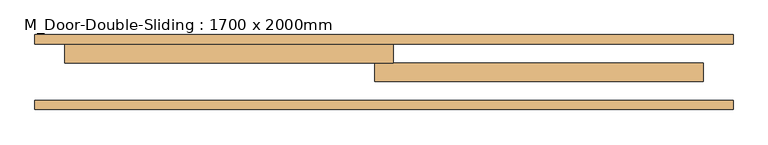
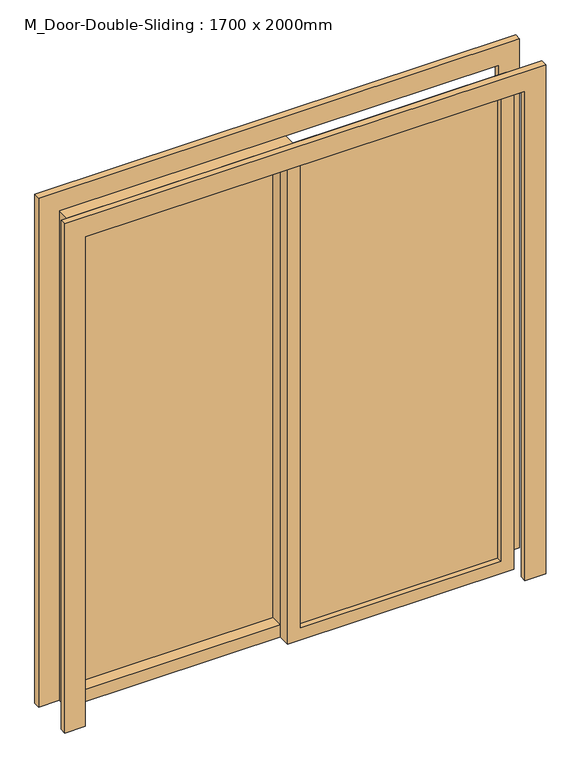
"""IFC4 building model written with IfcOpenShell, lengths in millimetres: door geometry, M_Door-Double-Sliding : 1700 x 2000mm."""

from ifc_helpers import new_model, si_unit, frame, origin, place, context, project, spatial, polyline, outline, extrude, source, transform, mapped, element, save


def m_door_double_sliding_1700_x_2000mm_d36f6dca(model_context):
    return source(origin(), model_context, "Body", "SweptSolid", [
        extrude(outline(polyline([(0.0, 930.0), (2080.0, 930.0), (2080.0, -930.0), (0.0, -930.0), (0.0, -850.0), (2000.0, -850.0), (2000.0, 850.0), (0.0, 850.0), (0.0, 930.0)])), frame((0.0, 202.0, 0.0), z_axis=(0.0, 1.0, 0.0), x_axis=(0.0, 0.0, 1.0)), (0.0, 0.0, 1.0), 25.0),
        extrude(outline(polyline([(0.0, -930.0), (0.0, -850.0), (2000.0, -850.0), (2000.0, 850.0), (0.0, 850.0), (0.0, 930.0), (2080.0, 930.0), (2080.0, -930.0), (0.0, -930.0)])), frame((0.0, 27.0, 0.0), z_axis=(0.0, 1.0, 0.0), x_axis=(0.0, 0.0, 1.0)), (0.0, 0.0, 1.0), 25.0),
        extrude(outline(polyline([(2000.0, 25.0), (2000.0, -850.0), (0.0, -850.0), (0.0, 25.0), (2000.0, 25.0)]), holes=[polyline([(1950.0, -25.0), (50.0, -25.0), (50.0, -800.0), (1950.0, -800.0), (1950.0, -25.0)])]), frame((0.0, 152.0, 0.0), z_axis=(0.0, 1.0, 0.0), x_axis=(0.0, 0.0, 1.0)), (0.0, 0.0, 1.0), 50.0),
        extrude(outline(polyline([(2000.0, -25.0), (0.0, -25.0), (0.0, 850.0), (2000.0, 850.0), (2000.0, -25.0)]), holes=[polyline([(1950.0, 25.0), (1950.0, 800.0), (50.0, 800.0), (50.0, 25.0), (1950.0, 25.0)])]), frame((0.0, 102.0, 0.0), z_axis=(0.0, 1.0, 0.0), x_axis=(0.0, 0.0, 1.0)), (0.0, 0.0, 1.0), 50.0),
        extrude(outline(polyline([(-25.0, 200.025), (-800.0, 200.025), (-800.0, 206.375), (-25.0, 206.375), (-25.0, 200.025)])), frame((0.0, 0.0, 50.0), z_axis=(0.0, 0.0, 1.0), x_axis=(1.0, 0.0, 0.0)), (0.0, 0.0, 1.0), 1900.0),
        extrude(outline(polyline([(25.0, 130.175), (800.0, 130.175), (800.0, 123.825), (25.0, 123.825), (25.0, 130.175)])), frame((0.0, 0.0, 50.0), z_axis=(0.0, 0.0, 1.0), x_axis=(1.0, 0.0, 0.0)), (0.0, 0.0, 1.0), 1900.0),
    ])


if __name__ == "__main__":
    model = new_model("IFC4")
    model_context = context("Model", 3, world=origin())
    ifc_project = project(units=[si_unit("LENGTHUNIT", "METRE", prefix="MILLI")], contexts=[model_context])
    site = spatial("IfcSite", under=ifc_project)
    building = spatial("IfcBuilding", under=site)
    placement = place(None, origin())
    m_door_double_sliding_1700_x_2000mm_shape = m_door_double_sliding_1700_x_2000mm_d36f6dca(model_context)
    element("IfcDoor", 1, ObjectType="M_Door-Double-Sliding : 1700 x 2000mm", at=placement, inside=building, context=model_context, shape_type="MappedRepresentation", body=[
        mapped(m_door_double_sliding_1700_x_2000mm_shape, transform((0.0, 0.0, 0.0), x_axis=(1.0, 0.0, 0.0), y_axis=(0.0, 1.0, 0.0), z_axis=(0.0, 0.0, 1.0))),
    ])
    save(model, "model.ifc")

# Revit data of these elements
# Type "M_Door-Double-Sliding : 1700 x 2000mm"
#   Type Mark = "40"
#   Construction Type Id = "opn-d45"
#   Assembly Code = "C1020"
#   Analytic Construction = "Wood frame, double glass door "
#   Thickness = 50 mm
#   Thermal Resistance (R) = 0.31964 (m²·K)/W
#   Heat Transfer Coefficient (U) = 3.12872 W/(m²·K)
#   Height = 2000 mm
#   Rail Width = 50 mm
#   Stiles = 50 mm
#   Trim Projection Ext = 25 mm
#   Trim Projection Int = 25 mm
#   Trim Width = 80 mm
#   Width = 1700 mm
#   Define Thermal Properties by = 1
#   Glazing = Glass
#   Panel Material = Wood - Birch - Solid Stained Light Low Gloss
#   Trim Material = Paint - Sienna
#   Visual Light Transmittance = 0
#   Solar Heat Gain Coefficient = 0
#   Function = (empty or 0)
#   Wall Closure = (empty or 0)
# Element 1 (IfcDoor, "M_Door-Double-Sliding : 1700 x 2000mm")
#   Materials on its faces: "Paint - Sienna", "Wood - Birch - Solid Stained Light Low Gloss", "Glass"
# Materials
#   "Glass": class "Glass", colour RGB 0 128 192, transparency 0.9, Description = "Soda Lime Glass", Cost = 0
#   "Wood - Birch - Solid Stained Light Low Gloss": class "Wood", colour RGB 210 159 95, transparency 0, Cost = 0
#   "Paint - Sienna": colour RGB 118 70 51, transparency 0, Cost = 0
